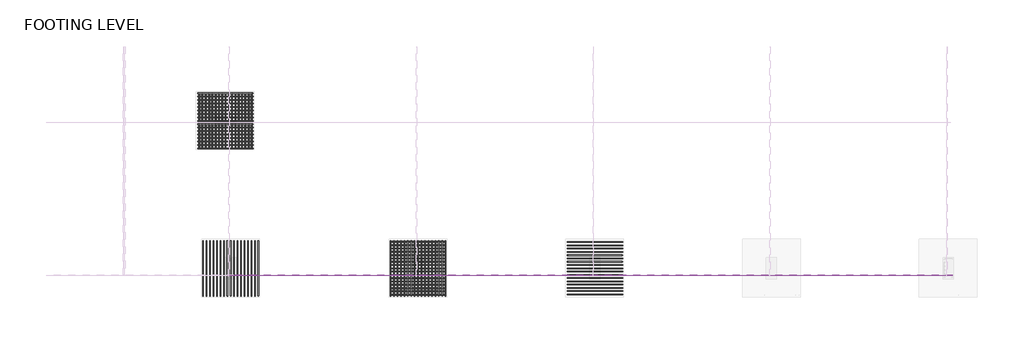
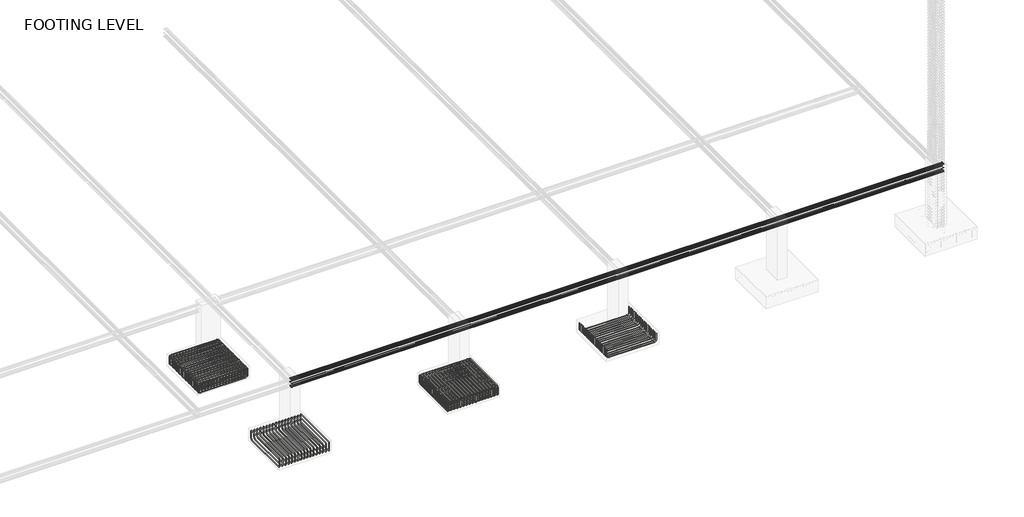
# One storey, part 5 of 19: 14 reinforcing bars.
"""IFC4 building model written with IfcOpenShell, lengths in millimetres."""

from ifc_helpers import new_model, si_unit, point, frame, origin, place, context, project, spatial, polyline, circle_curve, trimmed, segment, composite_curve, source, transform, mapped, element, save
from ifc_brep_helpers import swept_disk

model = new_model("IFC4")

# Units and contexts
model_context = context("Model", 3, world=origin())
ifc_project = project(units=[si_unit("LENGTHUNIT", "METRE", prefix="MILLI")], contexts=[model_context])

# Site, building, storey
site = spatial("IfcSite", under=ifc_project)
building = spatial("IfcBuilding", under=site)
storey = spatial("IfcBuildingStorey", under=building, Name="FOOTING LEVEL", Elevation=-3048.0)

# Reinforcing bars
placement = place(None, origin())
reinforcing_bar_shape = source(origin(), model_context, "Body", "SolidModel", [
    swept_disk(composite_curve([segment(polyline([(18259.8587563, -28952.7516566, -3148.0), (18259.8587563, -28952.7516566, -3470.1)]), True, "CONTINUOUS"), segment(trimmed(circle_curve(frame((18169.6587563, -28952.7516566, -3470.1), z_axis=(0.0, 1.0, 0.0), x_axis=(90.20000000000073, 0.0, 0.0)), 90.2), [point((18259.8587563, -28952.7516566, -3470.1))], [point((18169.6587563, -28952.7516566, -3560.3))], True, "CARTESIAN"), True, "CONTINUOUS"), segment(polyline([(18169.6587563, -28952.7516566, -3560.3), (15975.4587563, -28952.7516566, -3560.3)]), True, "CONTINUOUS"), segment(trimmed(circle_curve(frame((15975.4587563, -28952.7516566, -3470.1), z_axis=(0.0, 1.0, 0.0), x_axis=(0.0, 0.0, -90.20000000000027)), 90.2), [point((15975.4587563, -28952.7516566, -3560.3))], [point((15885.2587563, -28952.7516566, -3470.1))], True, "CARTESIAN"), True, "CONTINUOUS"), segment(polyline([(15885.2587563, -28952.7516566, -3470.1), (15885.2587563, -28952.7516566, -3148.0)]), True, "CONTINUOUS")], self_intersect=False), 12.7),
])
element("IfcReinforcingBar", 1, at=placement, inside=storey, context=model_context, shape_type="MappedRepresentation", body=[
    mapped(reinforcing_bar_shape, transform((0.0, 0.0, 0.0), x_axis=(1.0, 0.0, 0.0), y_axis=(0.0, 1.0, 0.0), z_axis=(0.0, 0.0, 1.0))),
    mapped(reinforcing_bar_shape, transform((0.0, 140.8090411, 0.0), x_axis=(1.0, 0.0, 0.0), y_axis=(0.0, 1.0, 0.0), z_axis=(0.0, 0.0, 1.0))),
    mapped(reinforcing_bar_shape, transform((0.0, 281.6180821, 0.0), x_axis=(1.0, 0.0, 0.0), y_axis=(0.0, 1.0, 0.0), z_axis=(0.0, 0.0, 1.0))),
    mapped(reinforcing_bar_shape, transform((0.0, 422.4271232, 0.0), x_axis=(1.0, 0.0, 0.0), y_axis=(0.0, 1.0, 0.0), z_axis=(0.0, 0.0, 1.0))),
    mapped(reinforcing_bar_shape, transform((0.0, 563.2361643, 0.0), x_axis=(1.0, 0.0, 0.0), y_axis=(0.0, 1.0, 0.0), z_axis=(0.0, 0.0, 1.0))),
    mapped(reinforcing_bar_shape, transform((0.0, 704.0452054, 0.0), x_axis=(1.0, 0.0, 0.0), y_axis=(0.0, 1.0, 0.0), z_axis=(0.0, 0.0, 1.0))),
    mapped(reinforcing_bar_shape, transform((0.0, 844.8542464, 0.0), x_axis=(1.0, 0.0, 0.0), y_axis=(0.0, 1.0, 0.0), z_axis=(0.0, 0.0, 1.0))),
    mapped(reinforcing_bar_shape, transform((0.0, 985.6632875, 0.0), x_axis=(1.0, 0.0, 0.0), y_axis=(0.0, 1.0, 0.0), z_axis=(0.0, 0.0, 1.0))),
    mapped(reinforcing_bar_shape, transform((0.0, 1126.4723286, 0.0), x_axis=(1.0, 0.0, 0.0), y_axis=(0.0, 1.0, 0.0), z_axis=(0.0, 0.0, 1.0))),
    mapped(reinforcing_bar_shape, transform((0.0, 1267.2813697, 0.0), x_axis=(1.0, 0.0, 0.0), y_axis=(0.0, 1.0, 0.0), z_axis=(0.0, 0.0, 1.0))),
    mapped(reinforcing_bar_shape, transform((0.0, 1408.0904107, 0.0), x_axis=(1.0, 0.0, 0.0), y_axis=(0.0, 1.0, 0.0), z_axis=(0.0, 0.0, 1.0))),
    mapped(reinforcing_bar_shape, transform((0.0, 1548.8994518, 0.0), x_axis=(1.0, 0.0, 0.0), y_axis=(0.0, 1.0, 0.0), z_axis=(0.0, 0.0, 1.0))),
    mapped(reinforcing_bar_shape, transform((0.0, 1689.7084929, 0.0), x_axis=(1.0, 0.0, 0.0), y_axis=(0.0, 1.0, 0.0), z_axis=(0.0, 0.0, 1.0))),
    mapped(reinforcing_bar_shape, transform((0.0, 1830.517534, 0.0), x_axis=(1.0, 0.0, 0.0), y_axis=(0.0, 1.0, 0.0), z_axis=(0.0, 0.0, 1.0))),
    mapped(reinforcing_bar_shape, transform((0.0, 1971.326575, 0.0), x_axis=(1.0, 0.0, 0.0), y_axis=(0.0, 1.0, 0.0), z_axis=(0.0, 0.0, 1.0))),
    mapped(reinforcing_bar_shape, transform((0.0, 2112.1356161, 0.0), x_axis=(1.0, 0.0, 0.0), y_axis=(0.0, 1.0, 0.0), z_axis=(0.0, 0.0, 1.0))),
    mapped(reinforcing_bar_shape, transform((0.0, 2252.9446572, 0.0), x_axis=(1.0, 0.0, 0.0), y_axis=(0.0, 1.0, 0.0), z_axis=(0.0, 0.0, 1.0))),
])
reinforcing_bar_2_shape = source(origin(), model_context, "Body", "SolidModel", [
    swept_disk(composite_curve([segment(polyline([(10639.8587563, -28952.7516566, -3148.0), (10639.8587563, -28952.7516566, -3470.1)]), True, "CONTINUOUS"), segment(trimmed(circle_curve(frame((10549.6587563, -28952.7516566, -3470.1), z_axis=(0.0, 1.0, 0.0), x_axis=(90.20000000000073, 0.0, 0.0)), 90.2), [point((10639.8587563, -28952.7516566, -3470.1))], [point((10549.6587563, -28952.7516566, -3560.3))], True, "CARTESIAN"), True, "CONTINUOUS"), segment(polyline([(10549.6587563, -28952.7516566, -3560.3), (8355.4587563, -28952.7516566, -3560.3)]), True, "CONTINUOUS"), segment(trimmed(circle_curve(frame((8355.4587563, -28952.7516566, -3470.1), z_axis=(0.0, 1.0, 0.0), x_axis=(0.0, 0.0, -90.20000000000027)), 90.2), [point((8355.4587563, -28952.7516566, -3560.3))], [point((8265.2587563, -28952.7516566, -3470.1))], True, "CARTESIAN"), True, "CONTINUOUS"), segment(polyline([(8265.2587563, -28952.7516566, -3470.1), (8265.2587563, -28952.7516566, -3148.0)]), True, "CONTINUOUS")], self_intersect=False), 12.7),
])
element("IfcReinforcingBar", 2, at=placement, inside=storey, context=model_context, shape_type="MappedRepresentation", body=[
    mapped(reinforcing_bar_2_shape, transform((0.0, 0.0, 0.0), x_axis=(1.0, 0.0, 0.0), y_axis=(0.0, 1.0, 0.0), z_axis=(0.0, 0.0, 1.0))),
    mapped(reinforcing_bar_2_shape, transform((0.0, 140.8090411, 0.0), x_axis=(1.0, 0.0, 0.0), y_axis=(0.0, 1.0, 0.0), z_axis=(0.0, 0.0, 1.0))),
    mapped(reinforcing_bar_2_shape, transform((0.0, 281.6180821, 0.0), x_axis=(1.0, 0.0, 0.0), y_axis=(0.0, 1.0, 0.0), z_axis=(0.0, 0.0, 1.0))),
    mapped(reinforcing_bar_2_shape, transform((0.0, 422.4271232, 0.0), x_axis=(1.0, 0.0, 0.0), y_axis=(0.0, 1.0, 0.0), z_axis=(0.0, 0.0, 1.0))),
    mapped(reinforcing_bar_2_shape, transform((0.0, 563.2361643, 0.0), x_axis=(1.0, 0.0, 0.0), y_axis=(0.0, 1.0, 0.0), z_axis=(0.0, 0.0, 1.0))),
    mapped(reinforcing_bar_2_shape, transform((0.0, 704.0452054, 0.0), x_axis=(1.0, 0.0, 0.0), y_axis=(0.0, 1.0, 0.0), z_axis=(0.0, 0.0, 1.0))),
    mapped(reinforcing_bar_2_shape, transform((0.0, 844.8542464, 0.0), x_axis=(1.0, 0.0, 0.0), y_axis=(0.0, 1.0, 0.0), z_axis=(0.0, 0.0, 1.0))),
    mapped(reinforcing_bar_2_shape, transform((0.0, 985.6632875, 0.0), x_axis=(1.0, 0.0, 0.0), y_axis=(0.0, 1.0, 0.0), z_axis=(0.0, 0.0, 1.0))),
    mapped(reinforcing_bar_2_shape, transform((0.0, 1126.4723286, 0.0), x_axis=(1.0, 0.0, 0.0), y_axis=(0.0, 1.0, 0.0), z_axis=(0.0, 0.0, 1.0))),
    mapped(reinforcing_bar_2_shape, transform((0.0, 1267.2813697, 0.0), x_axis=(1.0, 0.0, 0.0), y_axis=(0.0, 1.0, 0.0), z_axis=(0.0, 0.0, 1.0))),
    mapped(reinforcing_bar_2_shape, transform((0.0, 1408.0904107, 0.0), x_axis=(1.0, 0.0, 0.0), y_axis=(0.0, 1.0, 0.0), z_axis=(0.0, 0.0, 1.0))),
    mapped(reinforcing_bar_2_shape, transform((0.0, 1548.8994518, 0.0), x_axis=(1.0, 0.0, 0.0), y_axis=(0.0, 1.0, 0.0), z_axis=(0.0, 0.0, 1.0))),
    mapped(reinforcing_bar_2_shape, transform((0.0, 1689.7084929, 0.0), x_axis=(1.0, 0.0, 0.0), y_axis=(0.0, 1.0, 0.0), z_axis=(0.0, 0.0, 1.0))),
    mapped(reinforcing_bar_2_shape, transform((0.0, 1830.517534, 0.0), x_axis=(1.0, 0.0, 0.0), y_axis=(0.0, 1.0, 0.0), z_axis=(0.0, 0.0, 1.0))),
    mapped(reinforcing_bar_2_shape, transform((0.0, 1971.326575, 0.0), x_axis=(1.0, 0.0, 0.0), y_axis=(0.0, 1.0, 0.0), z_axis=(0.0, 0.0, 1.0))),
    mapped(reinforcing_bar_2_shape, transform((0.0, 2112.1356161, 0.0), x_axis=(1.0, 0.0, 0.0), y_axis=(0.0, 1.0, 0.0), z_axis=(0.0, 0.0, 1.0))),
    mapped(reinforcing_bar_2_shape, transform((0.0, 2252.9446572, 0.0), x_axis=(1.0, 0.0, 0.0), y_axis=(0.0, 1.0, 0.0), z_axis=(0.0, 0.0, 1.0))),
])
reinforcing_bar_3_shape = source(origin(), model_context, "Body", "SolidModel", [
    swept_disk(composite_curve([segment(polyline([(10639.8587563, -26677.3596072, -3548.0), (10639.8587563, -26677.3596072, -3225.9)]), True, "CONTINUOUS"), segment(trimmed(circle_curve(frame((10549.6587563, -26677.3596072, -3225.9), z_axis=(0.0, -1.0, 0.0), x_axis=(90.20000000000073, 0.0, 0.0)), 90.2), [point((10639.8587563, -26677.3596072, -3225.9))], [point((10549.6587563, -26677.3596072, -3135.7))], True, "CARTESIAN"), True, "CONTINUOUS"), segment(polyline([(10549.6587563, -26677.3596072, -3135.7), (8355.4587563, -26677.3596072, -3135.7)]), True, "CONTINUOUS"), segment(trimmed(circle_curve(frame((8355.4587563, -26677.3596072, -3225.9), z_axis=(0.0, -1.0, 0.0), x_axis=(0.0, 0.0, 90.20000000000027)), 90.2), [point((8355.4587563, -26677.3596072, -3135.7))], [point((8265.2587563, -26677.3596072, -3225.9))], True, "CARTESIAN"), True, "CONTINUOUS"), segment(polyline([(8265.2587563, -26677.3596072, -3225.9), (8265.2587563, -26677.3596072, -3548.0)]), True, "CONTINUOUS")], self_intersect=False), 12.7),
])
element("IfcReinforcingBar", 3, at=placement, inside=storey, context=model_context, shape_type="MappedRepresentation", body=[
    mapped(reinforcing_bar_3_shape, transform((0.0, 0.0, 0.0), x_axis=(1.0, 0.0, 0.0), y_axis=(0.0, 1.0, 0.0), z_axis=(0.0, 0.0, 1.0))),
    mapped(reinforcing_bar_3_shape, transform((0.0, -143.8496077, 0.0), x_axis=(1.0, 0.0, 0.0), y_axis=(0.0, 1.0, 0.0), z_axis=(0.0, 0.0, 1.0))),
    mapped(reinforcing_bar_3_shape, transform((0.0, -287.6992155, 0.0), x_axis=(1.0, 0.0, 0.0), y_axis=(0.0, 1.0, 0.0), z_axis=(0.0, 0.0, 1.0))),
    mapped(reinforcing_bar_3_shape, transform((0.0, -431.5488232, 0.0), x_axis=(1.0, 0.0, 0.0), y_axis=(0.0, 1.0, 0.0), z_axis=(0.0, 0.0, 1.0))),
    mapped(reinforcing_bar_3_shape, transform((0.0, -575.398431, 0.0), x_axis=(1.0, 0.0, 0.0), y_axis=(0.0, 1.0, 0.0), z_axis=(0.0, 0.0, 1.0))),
    mapped(reinforcing_bar_3_shape, transform((0.0, -719.2480387, 0.0), x_axis=(1.0, 0.0, 0.0), y_axis=(0.0, 1.0, 0.0), z_axis=(0.0, 0.0, 1.0))),
    mapped(reinforcing_bar_3_shape, transform((0.0, -863.0976465, 0.0), x_axis=(1.0, 0.0, 0.0), y_axis=(0.0, 1.0, 0.0), z_axis=(0.0, 0.0, 1.0))),
    mapped(reinforcing_bar_3_shape, transform((0.0, -1006.9472542, 0.0), x_axis=(1.0, 0.0, 0.0), y_axis=(0.0, 1.0, 0.0), z_axis=(0.0, 0.0, 1.0))),
    mapped(reinforcing_bar_3_shape, transform((0.0, -1150.796862, 0.0), x_axis=(1.0, 0.0, 0.0), y_axis=(0.0, 1.0, 0.0), z_axis=(0.0, 0.0, 1.0))),
    mapped(reinforcing_bar_3_shape, transform((0.0, -1294.6464697, 0.0), x_axis=(1.0, 0.0, 0.0), y_axis=(0.0, 1.0, 0.0), z_axis=(0.0, 0.0, 1.0))),
    mapped(reinforcing_bar_3_shape, transform((0.0, -1438.4960775, 0.0), x_axis=(1.0, 0.0, 0.0), y_axis=(0.0, 1.0, 0.0), z_axis=(0.0, 0.0, 1.0))),
    mapped(reinforcing_bar_3_shape, transform((0.0, -1582.3456852, 0.0), x_axis=(1.0, 0.0, 0.0), y_axis=(0.0, 1.0, 0.0), z_axis=(0.0, 0.0, 1.0))),
    mapped(reinforcing_bar_3_shape, transform((0.0, -1726.195293, 0.0), x_axis=(1.0, 0.0, 0.0), y_axis=(0.0, 1.0, 0.0), z_axis=(0.0, 0.0, 1.0))),
    mapped(reinforcing_bar_3_shape, transform((0.0, -1870.0449007, 0.0), x_axis=(1.0, 0.0, 0.0), y_axis=(0.0, 1.0, 0.0), z_axis=(0.0, 0.0, 1.0))),
    mapped(reinforcing_bar_3_shape, transform((0.0, -2013.8945085, 0.0), x_axis=(1.0, 0.0, 0.0), y_axis=(0.0, 1.0, 0.0), z_axis=(0.0, 0.0, 1.0))),
    mapped(reinforcing_bar_3_shape, transform((0.0, -2157.7441162, 0.0), x_axis=(1.0, 0.0, 0.0), y_axis=(0.0, 1.0, 0.0), z_axis=(0.0, 0.0, 1.0))),
    mapped(reinforcing_bar_3_shape, transform((0.0, -2301.5937239, 0.0), x_axis=(1.0, 0.0, 0.0), y_axis=(0.0, 1.0, 0.0), z_axis=(0.0, 0.0, 1.0))),
])
reinforcing_bar_4_shape = source(origin(), model_context, "Body", "SolidModel", [
    swept_disk(composite_curve([segment(polyline([(8265.2587563, -29018.3205555, -3173.0), (8265.2587563, -29018.3205555, -3495.1)]), True, "CONTINUOUS"), segment(trimmed(circle_curve(frame((8265.2587563, -28928.1205555, -3495.1), z_axis=(1.0, 0.0, 0.0), x_axis=(0.0, -90.19999999999709, 0.0)), 90.2), [point((8265.2587563, -29018.3205555, -3495.1))], [point((8265.2587563, -28928.1205555, -3585.3))], True, "CARTESIAN"), True, "CONTINUOUS"), segment(polyline([(8265.2587563, -28928.1205555, -3585.3), (8265.2587563, -26733.9205555, -3585.3)]), True, "CONTINUOUS"), segment(trimmed(circle_curve(frame((8265.2587563, -26733.9205555, -3495.1), z_axis=(1.0, 0.0, 0.0), x_axis=(0.0, 0.0, -90.20000000000027)), 90.2), [point((8265.2587563, -26733.9205555, -3585.3))], [point((8265.2587563, -26643.7205555, -3495.1))], True, "CARTESIAN"), True, "CONTINUOUS"), segment(polyline([(8265.2587563, -26643.7205555, -3495.1), (8265.2587563, -26643.7205555, -3173.0)]), True, "CONTINUOUS")], self_intersect=False), 12.7),
])
element("IfcReinforcingBar", 4, at=placement, inside=storey, context=model_context, shape_type="MappedRepresentation", body=[
    mapped(reinforcing_bar_4_shape, transform((0.0, 0.0, 0.0), x_axis=(1.0, 0.0, 0.0), y_axis=(0.0, 1.0, 0.0), z_axis=(0.0, 0.0, 1.0))),
    mapped(reinforcing_bar_4_shape, transform((148.4125, 0.0, 0.0), x_axis=(1.0, 0.0, 0.0), y_axis=(0.0, 1.0, 0.0), z_axis=(0.0, 0.0, 1.0))),
    mapped(reinforcing_bar_4_shape, transform((296.825, 0.0, 0.0), x_axis=(1.0, 0.0, 0.0), y_axis=(0.0, 1.0, 0.0), z_axis=(0.0, 0.0, 1.0))),
    mapped(reinforcing_bar_4_shape, transform((445.2375, 0.0, 0.0), x_axis=(1.0, 0.0, 0.0), y_axis=(0.0, 1.0, 0.0), z_axis=(0.0, 0.0, 1.0))),
    mapped(reinforcing_bar_4_shape, transform((593.65, 0.0, 0.0), x_axis=(1.0, 0.0, 0.0), y_axis=(0.0, 1.0, 0.0), z_axis=(0.0, 0.0, 1.0))),
    mapped(reinforcing_bar_4_shape, transform((742.0625, 0.0, 0.0), x_axis=(1.0, 0.0, 0.0), y_axis=(0.0, 1.0, 0.0), z_axis=(0.0, 0.0, 1.0))),
    mapped(reinforcing_bar_4_shape, transform((890.475, 0.0, 0.0), x_axis=(1.0, 0.0, 0.0), y_axis=(0.0, 1.0, 0.0), z_axis=(0.0, 0.0, 1.0))),
    mapped(reinforcing_bar_4_shape, transform((1038.8875, 0.0, 0.0), x_axis=(1.0, 0.0, 0.0), y_axis=(0.0, 1.0, 0.0), z_axis=(0.0, 0.0, 1.0))),
    mapped(reinforcing_bar_4_shape, transform((1187.3, 0.0, 0.0), x_axis=(1.0, 0.0, 0.0), y_axis=(0.0, 1.0, 0.0), z_axis=(0.0, 0.0, 1.0))),
    mapped(reinforcing_bar_4_shape, transform((1335.7125, 0.0, 0.0), x_axis=(1.0, 0.0, 0.0), y_axis=(0.0, 1.0, 0.0), z_axis=(0.0, 0.0, 1.0))),
    mapped(reinforcing_bar_4_shape, transform((1484.125, 0.0, 0.0), x_axis=(1.0, 0.0, 0.0), y_axis=(0.0, 1.0, 0.0), z_axis=(0.0, 0.0, 1.0))),
    mapped(reinforcing_bar_4_shape, transform((1632.5375, 0.0, 0.0), x_axis=(1.0, 0.0, 0.0), y_axis=(0.0, 1.0, 0.0), z_axis=(0.0, 0.0, 1.0))),
    mapped(reinforcing_bar_4_shape, transform((1780.95, 0.0, 0.0), x_axis=(1.0, 0.0, 0.0), y_axis=(0.0, 1.0, 0.0), z_axis=(0.0, 0.0, 1.0))),
    mapped(reinforcing_bar_4_shape, transform((1929.3625, 0.0, 0.0), x_axis=(1.0, 0.0, 0.0), y_axis=(0.0, 1.0, 0.0), z_axis=(0.0, 0.0, 1.0))),
    mapped(reinforcing_bar_4_shape, transform((2077.775, 0.0, 0.0), x_axis=(1.0, 0.0, 0.0), y_axis=(0.0, 1.0, 0.0), z_axis=(0.0, 0.0, 1.0))),
    mapped(reinforcing_bar_4_shape, transform((2226.1875, 0.0, 0.0), x_axis=(1.0, 0.0, 0.0), y_axis=(0.0, 1.0, 0.0), z_axis=(0.0, 0.0, 1.0))),
    mapped(reinforcing_bar_4_shape, transform((2374.6, 0.0, 0.0), x_axis=(1.0, 0.0, 0.0), y_axis=(0.0, 1.0, 0.0), z_axis=(0.0, 0.0, 1.0))),
])
reinforcing_bar_5_shape = source(origin(), model_context, "Body", "SolidModel", [
    swept_disk(composite_curve([segment(polyline([(8265.2587563, -26643.7205555, -3523.0), (8265.2587563, -26643.7205555, -3200.9)]), True, "CONTINUOUS"), segment(trimmed(circle_curve(frame((8265.2587563, -26733.9205555, -3200.9), z_axis=(1.0, 0.0, 0.0), x_axis=(0.0, 90.20000000000073, 0.0)), 90.2), [point((8265.2587563, -26643.7205555, -3200.9))], [point((8265.2587563, -26733.9205555, -3110.7))], True, "CARTESIAN"), True, "CONTINUOUS"), segment(polyline([(8265.2587563, -26733.9205555, -3110.7), (8265.2587563, -28928.1205555, -3110.7)]), True, "CONTINUOUS"), segment(trimmed(circle_curve(frame((8265.2587563, -28928.1205555, -3200.9), z_axis=(1.0, 0.0, 0.0), x_axis=(0.0, 0.0, 90.20000000000027)), 90.2), [point((8265.2587563, -28928.1205555, -3110.7))], [point((8265.2587563, -29018.3205555, -3200.9))], True, "CARTESIAN"), True, "CONTINUOUS"), segment(polyline([(8265.2587563, -29018.3205555, -3200.9), (8265.2587563, -29018.3205555, -3523.0)]), True, "CONTINUOUS")], self_intersect=False), 12.7),
])
element("IfcReinforcingBar", 5, at=placement, inside=storey, context=model_context, shape_type="MappedRepresentation", body=[
    mapped(reinforcing_bar_5_shape, transform((0.0, 0.0, 0.0), x_axis=(1.0, 0.0, 0.0), y_axis=(0.0, 1.0, 0.0), z_axis=(0.0, 0.0, 1.0))),
    mapped(reinforcing_bar_5_shape, transform((148.4125, 0.0, 0.0), x_axis=(1.0, 0.0, 0.0), y_axis=(0.0, 1.0, 0.0), z_axis=(0.0, 0.0, 1.0))),
    mapped(reinforcing_bar_5_shape, transform((296.825, 0.0, 0.0), x_axis=(1.0, 0.0, 0.0), y_axis=(0.0, 1.0, 0.0), z_axis=(0.0, 0.0, 1.0))),
    mapped(reinforcing_bar_5_shape, transform((445.2375, 0.0, 0.0), x_axis=(1.0, 0.0, 0.0), y_axis=(0.0, 1.0, 0.0), z_axis=(0.0, 0.0, 1.0))),
    mapped(reinforcing_bar_5_shape, transform((593.65, 0.0, 0.0), x_axis=(1.0, 0.0, 0.0), y_axis=(0.0, 1.0, 0.0), z_axis=(0.0, 0.0, 1.0))),
    mapped(reinforcing_bar_5_shape, transform((742.0625, 0.0, 0.0), x_axis=(1.0, 0.0, 0.0), y_axis=(0.0, 1.0, 0.0), z_axis=(0.0, 0.0, 1.0))),
    mapped(reinforcing_bar_5_shape, transform((890.475, 0.0, 0.0), x_axis=(1.0, 0.0, 0.0), y_axis=(0.0, 1.0, 0.0), z_axis=(0.0, 0.0, 1.0))),
    mapped(reinforcing_bar_5_shape, transform((1038.8875, 0.0, 0.0), x_axis=(1.0, 0.0, 0.0), y_axis=(0.0, 1.0, 0.0), z_axis=(0.0, 0.0, 1.0))),
    mapped(reinforcing_bar_5_shape, transform((1187.3, 0.0, 0.0), x_axis=(1.0, 0.0, 0.0), y_axis=(0.0, 1.0, 0.0), z_axis=(0.0, 0.0, 1.0))),
    mapped(reinforcing_bar_5_shape, transform((1335.7125, 0.0, 0.0), x_axis=(1.0, 0.0, 0.0), y_axis=(0.0, 1.0, 0.0), z_axis=(0.0, 0.0, 1.0))),
    mapped(reinforcing_bar_5_shape, transform((1484.125, 0.0, 0.0), x_axis=(1.0, 0.0, 0.0), y_axis=(0.0, 1.0, 0.0), z_axis=(0.0, 0.0, 1.0))),
    mapped(reinforcing_bar_5_shape, transform((1632.5375, 0.0, 0.0), x_axis=(1.0, 0.0, 0.0), y_axis=(0.0, 1.0, 0.0), z_axis=(0.0, 0.0, 1.0))),
    mapped(reinforcing_bar_5_shape, transform((1780.95, 0.0, 0.0), x_axis=(1.0, 0.0, 0.0), y_axis=(0.0, 1.0, 0.0), z_axis=(0.0, 0.0, 1.0))),
    mapped(reinforcing_bar_5_shape, transform((1929.3625, 0.0, 0.0), x_axis=(1.0, 0.0, 0.0), y_axis=(0.0, 1.0, 0.0), z_axis=(0.0, 0.0, 1.0))),
    mapped(reinforcing_bar_5_shape, transform((2077.775, 0.0, 0.0), x_axis=(1.0, 0.0, 0.0), y_axis=(0.0, 1.0, 0.0), z_axis=(0.0, 0.0, 1.0))),
    mapped(reinforcing_bar_5_shape, transform((2226.1875, 0.0, 0.0), x_axis=(1.0, 0.0, 0.0), y_axis=(0.0, 1.0, 0.0), z_axis=(0.0, 0.0, 1.0))),
    mapped(reinforcing_bar_5_shape, transform((2374.6, 0.0, 0.0), x_axis=(1.0, 0.0, 0.0), y_axis=(0.0, 1.0, 0.0), z_axis=(0.0, 0.0, 1.0))),
])
reinforcing_bar_6_shape = source(origin(), model_context, "Body", "SolidModel", [
    swept_disk(composite_curve([segment(polyline([(188.0587563, -29018.3205555, -3173.0), (188.0587563, -29018.3205555, -3495.1)]), True, "CONTINUOUS"), segment(trimmed(circle_curve(frame((188.0587563, -28928.1205555, -3495.1), z_axis=(1.0, 0.0, 0.0), x_axis=(0.0, -90.19999999999709, 0.0)), 90.2), [point((188.0587563, -29018.3205555, -3495.1))], [point((188.0587563, -28928.1205555, -3585.3))], True, "CARTESIAN"), True, "CONTINUOUS"), segment(polyline([(188.0587563, -28928.1205555, -3585.3), (188.0587563, -26733.9205555, -3585.3)]), True, "CONTINUOUS"), segment(trimmed(circle_curve(frame((188.0587563, -26733.9205555, -3495.1), z_axis=(1.0, 0.0, 0.0), x_axis=(0.0, 0.0, -90.20000000000027)), 90.2), [point((188.0587563, -26733.9205555, -3585.3))], [point((188.0587563, -26643.7205555, -3495.1))], True, "CARTESIAN"), True, "CONTINUOUS"), segment(polyline([(188.0587563, -26643.7205555, -3495.1), (188.0587563, -26643.7205555, -3173.0)]), True, "CONTINUOUS")], self_intersect=False), 12.7),
])
element("IfcReinforcingBar", 6, at=placement, inside=storey, context=model_context, shape_type="MappedRepresentation", body=[
    mapped(reinforcing_bar_6_shape, transform((0.0, 0.0, 0.0), x_axis=(1.0, 0.0, 0.0), y_axis=(0.0, 1.0, 0.0), z_axis=(0.0, 0.0, 1.0))),
    mapped(reinforcing_bar_6_shape, transform((148.4125, 0.0, 0.0), x_axis=(1.0, 0.0, 0.0), y_axis=(0.0, 1.0, 0.0), z_axis=(0.0, 0.0, 1.0))),
    mapped(reinforcing_bar_6_shape, transform((296.825, 0.0, 0.0), x_axis=(1.0, 0.0, 0.0), y_axis=(0.0, 1.0, 0.0), z_axis=(0.0, 0.0, 1.0))),
    mapped(reinforcing_bar_6_shape, transform((445.2375, 0.0, 0.0), x_axis=(1.0, 0.0, 0.0), y_axis=(0.0, 1.0, 0.0), z_axis=(0.0, 0.0, 1.0))),
    mapped(reinforcing_bar_6_shape, transform((593.65, 0.0, 0.0), x_axis=(1.0, 0.0, 0.0), y_axis=(0.0, 1.0, 0.0), z_axis=(0.0, 0.0, 1.0))),
    mapped(reinforcing_bar_6_shape, transform((742.0625, 0.0, 0.0), x_axis=(1.0, 0.0, 0.0), y_axis=(0.0, 1.0, 0.0), z_axis=(0.0, 0.0, 1.0))),
    mapped(reinforcing_bar_6_shape, transform((890.475, 0.0, 0.0), x_axis=(1.0, 0.0, 0.0), y_axis=(0.0, 1.0, 0.0), z_axis=(0.0, 0.0, 1.0))),
    mapped(reinforcing_bar_6_shape, transform((1038.8875, 0.0, 0.0), x_axis=(1.0, 0.0, 0.0), y_axis=(0.0, 1.0, 0.0), z_axis=(0.0, 0.0, 1.0))),
    mapped(reinforcing_bar_6_shape, transform((1187.3, 0.0, 0.0), x_axis=(1.0, 0.0, 0.0), y_axis=(0.0, 1.0, 0.0), z_axis=(0.0, 0.0, 1.0))),
    mapped(reinforcing_bar_6_shape, transform((1335.7125, 0.0, 0.0), x_axis=(1.0, 0.0, 0.0), y_axis=(0.0, 1.0, 0.0), z_axis=(0.0, 0.0, 1.0))),
    mapped(reinforcing_bar_6_shape, transform((1484.125, 0.0, 0.0), x_axis=(1.0, 0.0, 0.0), y_axis=(0.0, 1.0, 0.0), z_axis=(0.0, 0.0, 1.0))),
    mapped(reinforcing_bar_6_shape, transform((1632.5375, 0.0, 0.0), x_axis=(1.0, 0.0, 0.0), y_axis=(0.0, 1.0, 0.0), z_axis=(0.0, 0.0, 1.0))),
    mapped(reinforcing_bar_6_shape, transform((1780.95, 0.0, 0.0), x_axis=(1.0, 0.0, 0.0), y_axis=(0.0, 1.0, 0.0), z_axis=(0.0, 0.0, 1.0))),
    mapped(reinforcing_bar_6_shape, transform((1929.3625, 0.0, 0.0), x_axis=(1.0, 0.0, 0.0), y_axis=(0.0, 1.0, 0.0), z_axis=(0.0, 0.0, 1.0))),
    mapped(reinforcing_bar_6_shape, transform((2077.775, 0.0, 0.0), x_axis=(1.0, 0.0, 0.0), y_axis=(0.0, 1.0, 0.0), z_axis=(0.0, 0.0, 1.0))),
    mapped(reinforcing_bar_6_shape, transform((2226.1875, 0.0, 0.0), x_axis=(1.0, 0.0, 0.0), y_axis=(0.0, 1.0, 0.0), z_axis=(0.0, 0.0, 1.0))),
    mapped(reinforcing_bar_6_shape, transform((2374.6, 0.0, 0.0), x_axis=(1.0, 0.0, 0.0), y_axis=(0.0, 1.0, 0.0), z_axis=(0.0, 0.0, 1.0))),
])
reinforcing_bar_7_shape = source(origin(), model_context, "Body", "SolidModel", [
    swept_disk(composite_curve([segment(polyline([(188.0587563, -26643.7205555, -3523.0), (188.0587563, -26643.7205555, -3200.9)]), True, "CONTINUOUS"), segment(trimmed(circle_curve(frame((188.0587563, -26733.9205555, -3200.9), z_axis=(1.0, 0.0, 0.0), x_axis=(0.0, 90.20000000000073, 0.0)), 90.2), [point((188.0587563, -26643.7205555, -3200.9))], [point((188.0587563, -26733.9205555, -3110.7))], True, "CARTESIAN"), True, "CONTINUOUS"), segment(polyline([(188.0587563, -26733.9205555, -3110.7), (188.0587563, -28928.1205555, -3110.7)]), True, "CONTINUOUS"), segment(trimmed(circle_curve(frame((188.0587563, -28928.1205555, -3200.9), z_axis=(1.0, 0.0, 0.0), x_axis=(0.0, 0.0, 90.20000000000027)), 90.2), [point((188.0587563, -28928.1205555, -3110.7))], [point((188.0587563, -29018.3205555, -3200.9))], True, "CARTESIAN"), True, "CONTINUOUS"), segment(polyline([(188.0587563, -29018.3205555, -3200.9), (188.0587563, -29018.3205555, -3523.0)]), True, "CONTINUOUS")], self_intersect=False), 12.7),
])
element("IfcReinforcingBar", 7, at=placement, inside=storey, context=model_context, shape_type="MappedRepresentation", body=[
    mapped(reinforcing_bar_7_shape, transform((0.0, 0.0, 0.0), x_axis=(1.0, 0.0, 0.0), y_axis=(0.0, 1.0, 0.0), z_axis=(0.0, 0.0, 1.0))),
    mapped(reinforcing_bar_7_shape, transform((148.4125, 0.0, 0.0), x_axis=(1.0, 0.0, 0.0), y_axis=(0.0, 1.0, 0.0), z_axis=(0.0, 0.0, 1.0))),
    mapped(reinforcing_bar_7_shape, transform((296.825, 0.0, 0.0), x_axis=(1.0, 0.0, 0.0), y_axis=(0.0, 1.0, 0.0), z_axis=(0.0, 0.0, 1.0))),
    mapped(reinforcing_bar_7_shape, transform((445.2375, 0.0, 0.0), x_axis=(1.0, 0.0, 0.0), y_axis=(0.0, 1.0, 0.0), z_axis=(0.0, 0.0, 1.0))),
    mapped(reinforcing_bar_7_shape, transform((593.65, 0.0, 0.0), x_axis=(1.0, 0.0, 0.0), y_axis=(0.0, 1.0, 0.0), z_axis=(0.0, 0.0, 1.0))),
    mapped(reinforcing_bar_7_shape, transform((742.0625, 0.0, 0.0), x_axis=(1.0, 0.0, 0.0), y_axis=(0.0, 1.0, 0.0), z_axis=(0.0, 0.0, 1.0))),
    mapped(reinforcing_bar_7_shape, transform((890.475, 0.0, 0.0), x_axis=(1.0, 0.0, 0.0), y_axis=(0.0, 1.0, 0.0), z_axis=(0.0, 0.0, 1.0))),
    mapped(reinforcing_bar_7_shape, transform((1038.8875, 0.0, 0.0), x_axis=(1.0, 0.0, 0.0), y_axis=(0.0, 1.0, 0.0), z_axis=(0.0, 0.0, 1.0))),
    mapped(reinforcing_bar_7_shape, transform((1187.3, 0.0, 0.0), x_axis=(1.0, 0.0, 0.0), y_axis=(0.0, 1.0, 0.0), z_axis=(0.0, 0.0, 1.0))),
    mapped(reinforcing_bar_7_shape, transform((1335.7125, 0.0, 0.0), x_axis=(1.0, 0.0, 0.0), y_axis=(0.0, 1.0, 0.0), z_axis=(0.0, 0.0, 1.0))),
    mapped(reinforcing_bar_7_shape, transform((1484.125, 0.0, 0.0), x_axis=(1.0, 0.0, 0.0), y_axis=(0.0, 1.0, 0.0), z_axis=(0.0, 0.0, 1.0))),
    mapped(reinforcing_bar_7_shape, transform((1632.5375, 0.0, 0.0), x_axis=(1.0, 0.0, 0.0), y_axis=(0.0, 1.0, 0.0), z_axis=(0.0, 0.0, 1.0))),
    mapped(reinforcing_bar_7_shape, transform((1780.95, 0.0, 0.0), x_axis=(1.0, 0.0, 0.0), y_axis=(0.0, 1.0, 0.0), z_axis=(0.0, 0.0, 1.0))),
    mapped(reinforcing_bar_7_shape, transform((1929.3625, 0.0, 0.0), x_axis=(1.0, 0.0, 0.0), y_axis=(0.0, 1.0, 0.0), z_axis=(0.0, 0.0, 1.0))),
    mapped(reinforcing_bar_7_shape, transform((2077.775, 0.0, 0.0), x_axis=(1.0, 0.0, 0.0), y_axis=(0.0, 1.0, 0.0), z_axis=(0.0, 0.0, 1.0))),
    mapped(reinforcing_bar_7_shape, transform((2226.1875, 0.0, 0.0), x_axis=(1.0, 0.0, 0.0), y_axis=(0.0, 1.0, 0.0), z_axis=(0.0, 0.0, 1.0))),
    mapped(reinforcing_bar_7_shape, transform((2374.6, 0.0, 0.0), x_axis=(1.0, 0.0, 0.0), y_axis=(0.0, 1.0, 0.0), z_axis=(0.0, 0.0, 1.0))),
])
reinforcing_bar_8_shape = source(origin(), model_context, "Body", "SolidModel", [
    swept_disk(composite_curve([segment(polyline([(25.0276552, -22655.6205555, -3148.0), (25.0276552, -22655.6205555, -3470.1)]), True, "CONTINUOUS"), segment(trimmed(circle_curve(frame((25.0276552, -22565.4205555, -3470.1), z_axis=(1.0, 0.0, 0.0), x_axis=(0.0, -90.20000000000073, 0.0)), 90.2), [point((25.0276552, -22655.6205555, -3470.1))], [point((25.0276552, -22565.4205555, -3560.3))], True, "CARTESIAN"), True, "CONTINUOUS"), segment(polyline([(25.0276552, -22565.4205555, -3560.3), (25.0276552, -20371.2205555, -3560.3)]), True, "CONTINUOUS"), segment(trimmed(circle_curve(frame((25.0276552, -20371.2205555, -3470.1), z_axis=(1.0, 0.0, 0.0), x_axis=(0.0, 0.0, -90.20000000000027)), 90.2), [point((25.0276552, -20371.2205555, -3560.3))], [point((25.0276552, -20281.0205555, -3470.1))], True, "CARTESIAN"), True, "CONTINUOUS"), segment(polyline([(25.0276552, -20281.0205555, -3470.1), (25.0276552, -20281.0205555, -3148.0)]), True, "CONTINUOUS")], self_intersect=False), 12.7),
])
element("IfcReinforcingBar", 8, at=placement, inside=storey, context=model_context, shape_type="MappedRepresentation", body=[
    mapped(reinforcing_bar_8_shape, transform((0.0, 0.0, 0.0), x_axis=(1.0, 0.0, 0.0), y_axis=(0.0, 1.0, 0.0), z_axis=(0.0, 0.0, 1.0))),
    mapped(reinforcing_bar_8_shape, transform((140.8090411, 0.0, 0.0), x_axis=(1.0, 0.0, 0.0), y_axis=(0.0, 1.0, 0.0), z_axis=(0.0, 0.0, 1.0))),
    mapped(reinforcing_bar_8_shape, transform((281.6180821, 0.0, 0.0), x_axis=(1.0, 0.0, 0.0), y_axis=(0.0, 1.0, 0.0), z_axis=(0.0, 0.0, 1.0))),
    mapped(reinforcing_bar_8_shape, transform((422.4271232, 0.0, 0.0), x_axis=(1.0, 0.0, 0.0), y_axis=(0.0, 1.0, 0.0), z_axis=(0.0, 0.0, 1.0))),
    mapped(reinforcing_bar_8_shape, transform((563.2361643, 0.0, 0.0), x_axis=(1.0, 0.0, 0.0), y_axis=(0.0, 1.0, 0.0), z_axis=(0.0, 0.0, 1.0))),
    mapped(reinforcing_bar_8_shape, transform((704.0452054, 0.0, 0.0), x_axis=(1.0, 0.0, 0.0), y_axis=(0.0, 1.0, 0.0), z_axis=(0.0, 0.0, 1.0))),
    mapped(reinforcing_bar_8_shape, transform((844.8542464, 0.0, 0.0), x_axis=(1.0, 0.0, 0.0), y_axis=(0.0, 1.0, 0.0), z_axis=(0.0, 0.0, 1.0))),
    mapped(reinforcing_bar_8_shape, transform((985.6632875, 0.0, 0.0), x_axis=(1.0, 0.0, 0.0), y_axis=(0.0, 1.0, 0.0), z_axis=(0.0, 0.0, 1.0))),
    mapped(reinforcing_bar_8_shape, transform((1126.4723286, 0.0, 0.0), x_axis=(1.0, 0.0, 0.0), y_axis=(0.0, 1.0, 0.0), z_axis=(0.0, 0.0, 1.0))),
    mapped(reinforcing_bar_8_shape, transform((1267.2813697, 0.0, 0.0), x_axis=(1.0, 0.0, 0.0), y_axis=(0.0, 1.0, 0.0), z_axis=(0.0, 0.0, 1.0))),
    mapped(reinforcing_bar_8_shape, transform((1408.0904107, 0.0, 0.0), x_axis=(1.0, 0.0, 0.0), y_axis=(0.0, 1.0, 0.0), z_axis=(0.0, 0.0, 1.0))),
    mapped(reinforcing_bar_8_shape, transform((1548.8994518, 0.0, 0.0), x_axis=(1.0, 0.0, 0.0), y_axis=(0.0, 1.0, 0.0), z_axis=(0.0, 0.0, 1.0))),
    mapped(reinforcing_bar_8_shape, transform((1689.7084929, 0.0, 0.0), x_axis=(1.0, 0.0, 0.0), y_axis=(0.0, 1.0, 0.0), z_axis=(0.0, 0.0, 1.0))),
    mapped(reinforcing_bar_8_shape, transform((1830.517534, 0.0, 0.0), x_axis=(1.0, 0.0, 0.0), y_axis=(0.0, 1.0, 0.0), z_axis=(0.0, 0.0, 1.0))),
    mapped(reinforcing_bar_8_shape, transform((1971.326575, 0.0, 0.0), x_axis=(1.0, 0.0, 0.0), y_axis=(0.0, 1.0, 0.0), z_axis=(0.0, 0.0, 1.0))),
    mapped(reinforcing_bar_8_shape, transform((2112.1356161, 0.0, 0.0), x_axis=(1.0, 0.0, 0.0), y_axis=(0.0, 1.0, 0.0), z_axis=(0.0, 0.0, 1.0))),
    mapped(reinforcing_bar_8_shape, transform((2252.9446572, 0.0, 0.0), x_axis=(1.0, 0.0, 0.0), y_axis=(0.0, 1.0, 0.0), z_axis=(0.0, 0.0, 1.0))),
])
reinforcing_bar_9_shape = source(origin(), model_context, "Body", "SolidModel", [
    swept_disk(composite_curve([segment(polyline([(2300.4197045, -22655.6205555, -3548.0), (2300.4197045, -22655.6205555, -3225.9)]), True, "CONTINUOUS"), segment(trimmed(circle_curve(frame((2300.4197045, -22565.4205555, -3225.9), z_axis=(-1.0, 0.0, 0.0), x_axis=(0.0, -90.20000000000073, 0.0)), 90.2), [point((2300.4197045, -22655.6205555, -3225.9))], [point((2300.4197045, -22565.4205555, -3135.7))], True, "CARTESIAN"), True, "CONTINUOUS"), segment(polyline([(2300.4197045, -22565.4205555, -3135.7), (2300.4197045, -20371.2205555, -3135.7)]), True, "CONTINUOUS"), segment(trimmed(circle_curve(frame((2300.4197045, -20371.2205555, -3225.9), z_axis=(-1.0, 0.0, 0.0), x_axis=(0.0, 0.0, 90.20000000000027)), 90.2), [point((2300.4197045, -20371.2205555, -3135.7))], [point((2300.4197045, -20281.0205555, -3225.9))], True, "CARTESIAN"), True, "CONTINUOUS"), segment(polyline([(2300.4197045, -20281.0205555, -3225.9), (2300.4197045, -20281.0205555, -3548.0)]), True, "CONTINUOUS")], self_intersect=False), 12.7),
])
element("IfcReinforcingBar", 9, at=placement, inside=storey, context=model_context, shape_type="MappedRepresentation", body=[
    mapped(reinforcing_bar_9_shape, transform((0.0, 0.0, 0.0), x_axis=(1.0, 0.0, 0.0), y_axis=(0.0, 1.0, 0.0), z_axis=(0.0, 0.0, 1.0))),
    mapped(reinforcing_bar_9_shape, transform((-143.8496077, 0.0, 0.0), x_axis=(1.0, 0.0, 0.0), y_axis=(0.0, 1.0, 0.0), z_axis=(0.0, 0.0, 1.0))),
    mapped(reinforcing_bar_9_shape, transform((-287.6992155, 0.0, 0.0), x_axis=(1.0, 0.0, 0.0), y_axis=(0.0, 1.0, 0.0), z_axis=(0.0, 0.0, 1.0))),
    mapped(reinforcing_bar_9_shape, transform((-431.5488232, 0.0, 0.0), x_axis=(1.0, 0.0, 0.0), y_axis=(0.0, 1.0, 0.0), z_axis=(0.0, 0.0, 1.0))),
    mapped(reinforcing_bar_9_shape, transform((-575.398431, 0.0, 0.0), x_axis=(1.0, 0.0, 0.0), y_axis=(0.0, 1.0, 0.0), z_axis=(0.0, 0.0, 1.0))),
    mapped(reinforcing_bar_9_shape, transform((-719.2480387, 0.0, 0.0), x_axis=(1.0, 0.0, 0.0), y_axis=(0.0, 1.0, 0.0), z_axis=(0.0, 0.0, 1.0))),
    mapped(reinforcing_bar_9_shape, transform((-863.0976465, 0.0, 0.0), x_axis=(1.0, 0.0, 0.0), y_axis=(0.0, 1.0, 0.0), z_axis=(0.0, 0.0, 1.0))),
    mapped(reinforcing_bar_9_shape, transform((-1006.9472542, 0.0, 0.0), x_axis=(1.0, 0.0, 0.0), y_axis=(0.0, 1.0, 0.0), z_axis=(0.0, 0.0, 1.0))),
    mapped(reinforcing_bar_9_shape, transform((-1150.796862, 0.0, 0.0), x_axis=(1.0, 0.0, 0.0), y_axis=(0.0, 1.0, 0.0), z_axis=(0.0, 0.0, 1.0))),
    mapped(reinforcing_bar_9_shape, transform((-1294.6464697, 0.0, 0.0), x_axis=(1.0, 0.0, 0.0), y_axis=(0.0, 1.0, 0.0), z_axis=(0.0, 0.0, 1.0))),
    mapped(reinforcing_bar_9_shape, transform((-1438.4960775, 0.0, 0.0), x_axis=(1.0, 0.0, 0.0), y_axis=(0.0, 1.0, 0.0), z_axis=(0.0, 0.0, 1.0))),
    mapped(reinforcing_bar_9_shape, transform((-1582.3456852, 0.0, 0.0), x_axis=(1.0, 0.0, 0.0), y_axis=(0.0, 1.0, 0.0), z_axis=(0.0, 0.0, 1.0))),
    mapped(reinforcing_bar_9_shape, transform((-1726.195293, 0.0, 0.0), x_axis=(1.0, 0.0, 0.0), y_axis=(0.0, 1.0, 0.0), z_axis=(0.0, 0.0, 1.0))),
    mapped(reinforcing_bar_9_shape, transform((-1870.0449007, 0.0, 0.0), x_axis=(1.0, 0.0, 0.0), y_axis=(0.0, 1.0, 0.0), z_axis=(0.0, 0.0, 1.0))),
    mapped(reinforcing_bar_9_shape, transform((-2013.8945085, 0.0, 0.0), x_axis=(1.0, 0.0, 0.0), y_axis=(0.0, 1.0, 0.0), z_axis=(0.0, 0.0, 1.0))),
    mapped(reinforcing_bar_9_shape, transform((-2157.7441162, 0.0, 0.0), x_axis=(1.0, 0.0, 0.0), y_axis=(0.0, 1.0, 0.0), z_axis=(0.0, 0.0, 1.0))),
    mapped(reinforcing_bar_9_shape, transform((-2301.5937239, 0.0, 0.0), x_axis=(1.0, 0.0, 0.0), y_axis=(0.0, 1.0, 0.0), z_axis=(0.0, 0.0, 1.0))),
])
reinforcing_bar_10_shape = source(origin(), model_context, "Body", "SolidModel", [
    swept_disk(composite_curve([segment(polyline([(-40.5412437, -20281.0205555, -3173.0), (-40.5412437, -20281.0205555, -3495.1)]), True, "CONTINUOUS"), segment(trimmed(circle_curve(frame((49.6587563, -20281.0205555, -3495.1), z_axis=(0.0, -1.0, 0.0), x_axis=(-90.2, 0.0, 0.0)), 90.2), [point((-40.5412437, -20281.0205555, -3495.1))], [point((49.6587563, -20281.0205555, -3585.3))], True, "CARTESIAN"), True, "CONTINUOUS"), segment(polyline([(49.6587563, -20281.0205555, -3585.3), (2243.8587563, -20281.0205555, -3585.3)]), True, "CONTINUOUS"), segment(trimmed(circle_curve(frame((2243.8587563, -20281.0205555, -3495.1), z_axis=(0.0, -1.0, 0.0), x_axis=(0.0, 0.0, -90.20000000000027)), 90.2), [point((2243.8587563, -20281.0205555, -3585.3))], [point((2334.0587563, -20281.0205555, -3495.1))], True, "CARTESIAN"), True, "CONTINUOUS"), segment(polyline([(2334.0587563, -20281.0205555, -3495.1), (2334.0587563, -20281.0205555, -3173.0)]), True, "CONTINUOUS")], self_intersect=False), 12.7),
])
element("IfcReinforcingBar", 10, at=placement, inside=storey, context=model_context, shape_type="MappedRepresentation", body=[
    mapped(reinforcing_bar_10_shape, transform((0.0, 0.0, 0.0), x_axis=(1.0, 0.0, 0.0), y_axis=(0.0, 1.0, 0.0), z_axis=(0.0, 0.0, 1.0))),
    mapped(reinforcing_bar_10_shape, transform((0.0, -148.4125, 0.0), x_axis=(1.0, 0.0, 0.0), y_axis=(0.0, 1.0, 0.0), z_axis=(0.0, 0.0, 1.0))),
    mapped(reinforcing_bar_10_shape, transform((0.0, -296.825, 0.0), x_axis=(1.0, 0.0, 0.0), y_axis=(0.0, 1.0, 0.0), z_axis=(0.0, 0.0, 1.0))),
    mapped(reinforcing_bar_10_shape, transform((0.0, -445.2375, 0.0), x_axis=(1.0, 0.0, 0.0), y_axis=(0.0, 1.0, 0.0), z_axis=(0.0, 0.0, 1.0))),
    mapped(reinforcing_bar_10_shape, transform((0.0, -593.65, 0.0), x_axis=(1.0, 0.0, 0.0), y_axis=(0.0, 1.0, 0.0), z_axis=(0.0, 0.0, 1.0))),
    mapped(reinforcing_bar_10_shape, transform((0.0, -742.0625, 0.0), x_axis=(1.0, 0.0, 0.0), y_axis=(0.0, 1.0, 0.0), z_axis=(0.0, 0.0, 1.0))),
    mapped(reinforcing_bar_10_shape, transform((0.0, -890.475, 0.0), x_axis=(1.0, 0.0, 0.0), y_axis=(0.0, 1.0, 0.0), z_axis=(0.0, 0.0, 1.0))),
    mapped(reinforcing_bar_10_shape, transform((0.0, -1038.8875, 0.0), x_axis=(1.0, 0.0, 0.0), y_axis=(0.0, 1.0, 0.0), z_axis=(0.0, 0.0, 1.0))),
    mapped(reinforcing_bar_10_shape, transform((0.0, -1187.3, 0.0), x_axis=(1.0, 0.0, 0.0), y_axis=(0.0, 1.0, 0.0), z_axis=(0.0, 0.0, 1.0))),
    mapped(reinforcing_bar_10_shape, transform((0.0, -1335.7125, 0.0), x_axis=(1.0, 0.0, 0.0), y_axis=(0.0, 1.0, 0.0), z_axis=(0.0, 0.0, 1.0))),
    mapped(reinforcing_bar_10_shape, transform((0.0, -1484.125, 0.0), x_axis=(1.0, 0.0, 0.0), y_axis=(0.0, 1.0, 0.0), z_axis=(0.0, 0.0, 1.0))),
    mapped(reinforcing_bar_10_shape, transform((0.0, -1632.5375, 0.0), x_axis=(1.0, 0.0, 0.0), y_axis=(0.0, 1.0, 0.0), z_axis=(0.0, 0.0, 1.0))),
    mapped(reinforcing_bar_10_shape, transform((0.0, -1780.95, 0.0), x_axis=(1.0, 0.0, 0.0), y_axis=(0.0, 1.0, 0.0), z_axis=(0.0, 0.0, 1.0))),
    mapped(reinforcing_bar_10_shape, transform((0.0, -1929.3625, 0.0), x_axis=(1.0, 0.0, 0.0), y_axis=(0.0, 1.0, 0.0), z_axis=(0.0, 0.0, 1.0))),
    mapped(reinforcing_bar_10_shape, transform((0.0, -2077.775, 0.0), x_axis=(1.0, 0.0, 0.0), y_axis=(0.0, 1.0, 0.0), z_axis=(0.0, 0.0, 1.0))),
    mapped(reinforcing_bar_10_shape, transform((0.0, -2226.1875, 0.0), x_axis=(1.0, 0.0, 0.0), y_axis=(0.0, 1.0, 0.0), z_axis=(0.0, 0.0, 1.0))),
    mapped(reinforcing_bar_10_shape, transform((0.0, -2374.6, 0.0), x_axis=(1.0, 0.0, 0.0), y_axis=(0.0, 1.0, 0.0), z_axis=(0.0, 0.0, 1.0))),
])
reinforcing_bar_11_shape = source(origin(), model_context, "Body", "SolidModel", [
    swept_disk(composite_curve([segment(polyline([(2334.0587563, -20281.0205555, -3523.0), (2334.0587563, -20281.0205555, -3200.9)]), True, "CONTINUOUS"), segment(trimmed(circle_curve(frame((2243.8587563, -20281.0205555, -3200.9), z_axis=(0.0, -1.0, 0.0), x_axis=(90.19999999999982, 0.0, 0.0)), 90.2), [point((2334.0587563, -20281.0205555, -3200.9))], [point((2243.8587563, -20281.0205555, -3110.7))], True, "CARTESIAN"), True, "CONTINUOUS"), segment(polyline([(2243.8587563, -20281.0205555, -3110.7), (49.6587563, -20281.0205555, -3110.7)]), True, "CONTINUOUS"), segment(trimmed(circle_curve(frame((49.6587563, -20281.0205555, -3200.9), z_axis=(0.0, -1.0, 0.0), x_axis=(0.0, 0.0, 90.20000000000027)), 90.2), [point((49.6587563, -20281.0205555, -3110.7))], [point((-40.5412437, -20281.0205555, -3200.9))], True, "CARTESIAN"), True, "CONTINUOUS"), segment(polyline([(-40.5412437, -20281.0205555, -3200.9), (-40.5412437, -20281.0205555, -3523.0)]), True, "CONTINUOUS")], self_intersect=False), 12.7),
])
element("IfcReinforcingBar", 11, at=placement, inside=storey, context=model_context, shape_type="MappedRepresentation", body=[
    mapped(reinforcing_bar_11_shape, transform((0.0, 0.0, 0.0), x_axis=(1.0, 0.0, 0.0), y_axis=(0.0, 1.0, 0.0), z_axis=(0.0, 0.0, 1.0))),
    mapped(reinforcing_bar_11_shape, transform((0.0, -148.4125, 0.0), x_axis=(1.0, 0.0, 0.0), y_axis=(0.0, 1.0, 0.0), z_axis=(0.0, 0.0, 1.0))),
    mapped(reinforcing_bar_11_shape, transform((0.0, -296.825, 0.0), x_axis=(1.0, 0.0, 0.0), y_axis=(0.0, 1.0, 0.0), z_axis=(0.0, 0.0, 1.0))),
    mapped(reinforcing_bar_11_shape, transform((0.0, -445.2375, 0.0), x_axis=(1.0, 0.0, 0.0), y_axis=(0.0, 1.0, 0.0), z_axis=(0.0, 0.0, 1.0))),
    mapped(reinforcing_bar_11_shape, transform((0.0, -593.65, 0.0), x_axis=(1.0, 0.0, 0.0), y_axis=(0.0, 1.0, 0.0), z_axis=(0.0, 0.0, 1.0))),
    mapped(reinforcing_bar_11_shape, transform((0.0, -742.0625, 0.0), x_axis=(1.0, 0.0, 0.0), y_axis=(0.0, 1.0, 0.0), z_axis=(0.0, 0.0, 1.0))),
    mapped(reinforcing_bar_11_shape, transform((0.0, -890.475, 0.0), x_axis=(1.0, 0.0, 0.0), y_axis=(0.0, 1.0, 0.0), z_axis=(0.0, 0.0, 1.0))),
    mapped(reinforcing_bar_11_shape, transform((0.0, -1038.8875, 0.0), x_axis=(1.0, 0.0, 0.0), y_axis=(0.0, 1.0, 0.0), z_axis=(0.0, 0.0, 1.0))),
    mapped(reinforcing_bar_11_shape, transform((0.0, -1187.3, 0.0), x_axis=(1.0, 0.0, 0.0), y_axis=(0.0, 1.0, 0.0), z_axis=(0.0, 0.0, 1.0))),
    mapped(reinforcing_bar_11_shape, transform((0.0, -1335.7125, 0.0), x_axis=(1.0, 0.0, 0.0), y_axis=(0.0, 1.0, 0.0), z_axis=(0.0, 0.0, 1.0))),
    mapped(reinforcing_bar_11_shape, transform((0.0, -1484.125, 0.0), x_axis=(1.0, 0.0, 0.0), y_axis=(0.0, 1.0, 0.0), z_axis=(0.0, 0.0, 1.0))),
    mapped(reinforcing_bar_11_shape, transform((0.0, -1632.5375, 0.0), x_axis=(1.0, 0.0, 0.0), y_axis=(0.0, 1.0, 0.0), z_axis=(0.0, 0.0, 1.0))),
    mapped(reinforcing_bar_11_shape, transform((0.0, -1780.95, 0.0), x_axis=(1.0, 0.0, 0.0), y_axis=(0.0, 1.0, 0.0), z_axis=(0.0, 0.0, 1.0))),
    mapped(reinforcing_bar_11_shape, transform((0.0, -1929.3625, 0.0), x_axis=(1.0, 0.0, 0.0), y_axis=(0.0, 1.0, 0.0), z_axis=(0.0, 0.0, 1.0))),
    mapped(reinforcing_bar_11_shape, transform((0.0, -2077.775, 0.0), x_axis=(1.0, 0.0, 0.0), y_axis=(0.0, 1.0, 0.0), z_axis=(0.0, 0.0, 1.0))),
    mapped(reinforcing_bar_11_shape, transform((0.0, -2226.1875, 0.0), x_axis=(1.0, 0.0, 0.0), y_axis=(0.0, 1.0, 0.0), z_axis=(0.0, 0.0, 1.0))),
    mapped(reinforcing_bar_11_shape, transform((0.0, -2374.6, 0.0), x_axis=(1.0, 0.0, 0.0), y_axis=(0.0, 1.0, 0.0), z_axis=(0.0, 0.0, 1.0))),
])
reinforcing_bar_12_shape = source(origin(), model_context, "Body", "SolidModel", [
    swept_disk(composite_curve([segment(polyline([(32501.1587563, -27989.7999188, -412.7206367), (1260.2881621, -27989.7999188, -412.7206367)]), True, "CONTINUOUS")], self_intersect=False), 7.95),
])
element("IfcReinforcingBar", 12, at=placement, inside=storey, context=model_context, shape_type="MappedRepresentation", body=[
    mapped(reinforcing_bar_12_shape, transform((0.0, 0.0, 0.0), x_axis=(1.0, 0.0, 0.0), y_axis=(0.0, 1.0, 0.0), z_axis=(0.0, 0.0, 1.0))),
    mapped(reinforcing_bar_12_shape, transform((0.0, -69.8206367, 0.0), x_axis=(1.0, 0.0, 0.0), y_axis=(0.0, 1.0, 0.0), z_axis=(0.0, 0.0, 1.0))),
    mapped(reinforcing_bar_12_shape, transform((0.0, -139.6412734, 0.0), x_axis=(1.0, 0.0, 0.0), y_axis=(0.0, 1.0, 0.0), z_axis=(0.0, 0.0, 1.0))),
])
reinforcing_bar_13_shape = source(origin(), model_context, "Body", "SolidModel", [
    swept_disk(composite_curve([segment(polyline([(32501.1587563, -27989.7999188, -44.4793633), (1264.3907557, -27989.7999188, -44.4793633)]), True, "CONTINUOUS")], self_intersect=False), 7.95),
])
element("IfcReinforcingBar", 13, at=placement, inside=storey, context=model_context, shape_type="MappedRepresentation", body=[
    mapped(reinforcing_bar_13_shape, transform((0.0, 0.0, 0.0), x_axis=(1.0, 0.0, 0.0), y_axis=(0.0, 1.0, 0.0), z_axis=(0.0, 0.0, 1.0))),
    mapped(reinforcing_bar_13_shape, transform((0.0, -69.8206367, 0.0), x_axis=(1.0, 0.0, 0.0), y_axis=(0.0, 1.0, 0.0), z_axis=(0.0, 0.0, 1.0))),
    mapped(reinforcing_bar_13_shape, transform((0.0, -139.6412734, 0.0), x_axis=(1.0, 0.0, 0.0), y_axis=(0.0, 1.0, 0.0), z_axis=(0.0, 0.0, 1.0))),
])
reinforcing_bar_14_shape = source(origin(), model_context, "Body", "SolidModel", [
    swept_disk(composite_curve([segment(polyline([(32501.1587563, -28132.9705555, -228.3387181), (1264.839764, -28132.9705555, -228.3387181)]), True, "CONTINUOUS")], self_intersect=False), 7.95),
])
element("IfcReinforcingBar", 14, at=placement, inside=storey, context=model_context, shape_type="MappedRepresentation", body=[
    mapped(reinforcing_bar_14_shape, transform((0.0, 0.0, 0.0), x_axis=(1.0, 0.0, 0.0), y_axis=(0.0, 1.0, 0.0), z_axis=(0.0, 0.0, 1.0))),
    mapped(reinforcing_bar_14_shape, transform((0.0, 146.7, 0.0), x_axis=(1.0, 0.0, 0.0), y_axis=(0.0, 1.0, 0.0), z_axis=(0.0, 0.0, 1.0))),
])

save(model, "model.ifc")

# Revit data of these elements
# Elements 1, 2, 3, 4, 5, 6, 7, 8, 9, 10, 11, 12, 13, 14 (IfcReinforcingBar)
#   Phase Created = New Construction
